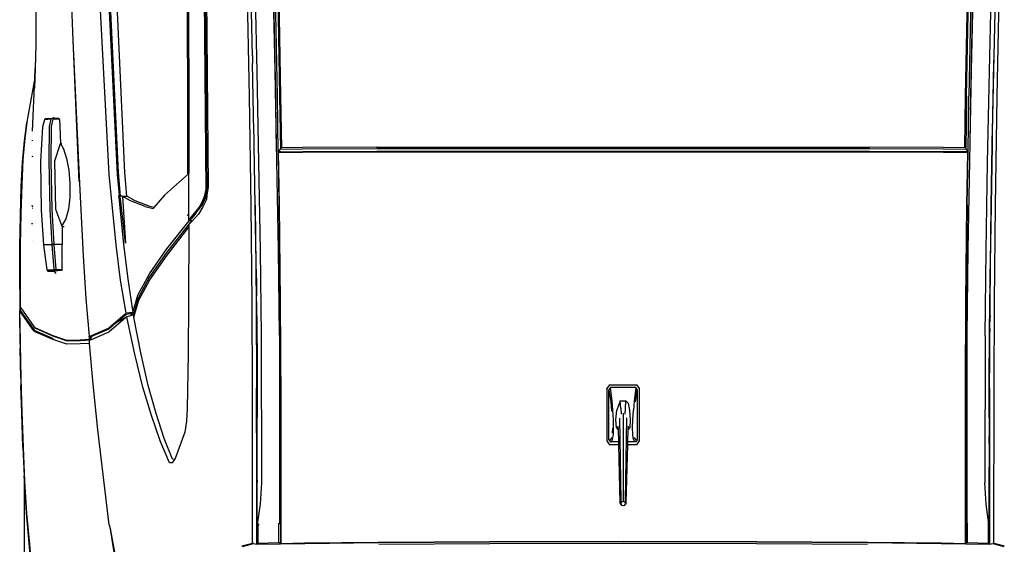
# Model space of a CAD drawing. Units: inches. Extents: x 22042254 to 25404563, y 17568978 to 17626777.
# Tile 26 of 45: x 22179810 to 22179874, y 17626227 to 17626261. Entities that reach past the tile are written whole.
import ezdxf

# ---------------------------------------------------------------- set-up
doc = ezdxf.new("R2010")
doc.units = ezdxf.units.IN
doc.header["$MEASUREMENT"] = 0
doc.layers.add('A-SITE-VEHI', color=8, linetype='Continuous', lineweight=18)
doc.layers.add('Edges', color=250, linetype='Continuous')

# ---------------------------------------------------------------- blocks, each defined once
blk = doc.blocks.new('Nissan Qashqai pl')
at = {"layer": 'Edges'}
for p, q in [((11.0581, 12.4738), (11.0614, 12.4872)), ((11.0582, 12.47), (11.0624, 12.4866)), ((10.3586, 12.4651), (10.2201, 12.4683)), ((10.2203, 12.4743), (10.3353, 12.4717)), ((10.2211, 12.4795), (10.3955, 12.4762)), ((10.3353, 12.4717), (10.4477, 12.4694)), ((10.3353, 12.4717), (10.346, 12.4714)), ((10.346, 12.4714), (10.4477, 12.4694)), ((10.3955, 12.4762), (10.5572, 12.4737)), ((10.4477, 12.4694), (10.4538, 12.4693)), ((10.4538, 12.4693), (10.4681, 12.469)), ((10.4676, 12.4691), (10.4538, 12.4693)), ((10.5566, 12.4677), (10.4676, 12.4691)), ((10.4676, 12.4691), (10.546, 12.4677)), ((10.4681, 12.469), (10.5866, 12.467)), ((10.546, 12.4677), (10.546, 12.4678)), ((10.546, 12.4677), (10.5576, 12.4675)), ((10.7, 12.4662), (10.5566, 12.4677)), ((10.5572, 12.4737), (10.7004, 12.4722)), ((10.5576, 12.4675), (10.6649, 12.4659)), ((10.5866, 12.467), (10.6649, 12.4659)), ((10.7004, 12.4722), (10.8279, 12.4715)), ((10.8279, 12.4715), (11.0544, 12.4714)), ((11.0544, 12.4714), (11.0575, 12.4714)), ((11.0575, 12.4714), (11.0581, 12.4738)), ((11.0575, 12.4714), (11.0582, 12.47)), ((11.0592, 12.4653), (11.0582, 12.47)), ((10.4931, 12.4624), (10.3586, 12.4651)), ((10.6237, 12.4603), (10.4931, 12.4624)), ((10.7502, 12.4586), (10.6237, 12.4603)), ((10.6649, 12.4659), (10.6786, 12.4658)), ((10.6649, 12.4659), (10.6772, 12.4657)), ((10.6786, 12.4657), (10.6772, 12.4657)), ((10.6786, 12.4658), (10.6786, 12.4662)), ((10.6786, 12.4657), (10.6786, 12.4658)), ((10.6786, 12.4658), (10.6801, 12.4657)), ((10.6786, 12.4657), (10.6801, 12.4657)), ((10.6801, 12.4662), (10.6801, 12.4657)), ((10.6801, 12.4657), (10.6801, 12.4657)), ((10.6801, 12.4657), (10.6811, 12.4657)), ((10.6801, 12.4657), (10.6811, 12.4657)), ((10.6811, 12.4662), (10.6811, 12.4657)), ((10.6811, 12.4657), (10.6811, 12.4657)), ((10.6811, 12.4657), (10.6966, 12.4654)), ((10.6811, 12.4657), (10.6991, 12.4655)), ((10.6811, 12.4657), (10.6991, 12.4655)), ((10.6966, 12.4654), (10.7144, 12.4653)), ((10.6991, 12.4655), (10.7144, 12.4653)), ((10.7201, 12.4661), (10.7, 12.4662)), ((10.7144, 12.4653), (10.7239, 12.4653)), ((10.7201, 12.4661), (10.7306, 12.4653)), ((10.7395, 12.4659), (10.7201, 12.4661)), ((10.7239, 12.4653), (10.7248, 12.4653)), ((10.7306, 12.4653), (10.7248, 12.4653)), ((10.7311, 12.4652), (10.7306, 12.4653)), ((10.7495, 12.4652), (10.7311, 12.4652)), ((10.7311, 12.4652), (10.7502, 12.4651)), ((10.7395, 12.4659), (10.7495, 12.4652)), ((10.7923, 12.4656), (10.7395, 12.4659)), ((10.8179, 12.4648), (10.7495, 12.4652)), ((10.7502, 12.4651), (10.7504, 12.4651)), ((10.7502, 12.4586), (10.968, 12.4585)), ((10.7504, 12.4651), (10.7808, 12.4649)), ((10.7808, 12.4649), (10.8179, 12.4648)), ((10.7923, 12.4652), (10.7923, 12.4656)), ((10.7933, 12.4656), (10.7923, 12.4656)), ((10.7933, 12.4652), (10.7933, 12.4656)), ((10.804, 12.4656), (10.7933, 12.4656)), ((10.804, 12.4653), (10.804, 12.4656)), ((10.8075, 12.4655), (10.804, 12.4656)), ((10.8075, 12.4655), (10.8075, 12.4653)), ((10.811, 12.4655), (10.8075, 12.4655)), ((10.811, 12.4655), (10.811, 12.4653)), ((10.8145, 12.4655), (10.811, 12.4655)), ((10.8145, 12.4653), (10.8145, 12.4655)), ((10.8279, 12.4654), (10.8145, 12.4655)), ((10.8277, 12.4647), (10.8179, 12.4648)), ((10.8711, 12.4646), (10.8277, 12.4647)), ((10.8279, 12.4654), (11.0592, 12.4653)), ((10.8711, 12.4646), (10.8824, 12.4646)), ((10.8824, 12.4646), (10.8825, 12.4646)), ((10.8825, 12.4646), (10.8884, 12.4646)), ((10.8884, 12.4646), (10.8923, 12.4646)), ((10.8923, 12.4646), (10.8996, 12.4646)), ((10.9097, 12.4646), (10.8996, 12.4646)), ((10.9097, 12.4646), (10.9399, 12.4646)), ((10.9399, 12.4646), (10.9491, 12.4645)), ((10.9491, 12.4645), (11.0301, 12.4645)), ((11, 12.4605), (10.968, 12.4585)), ((11.0301, 12.4645), (11, 12.4605)), ((11.0301, 12.4637), (11.0287, 12.4637)), ((11.03, 12.4635), (11.0301, 12.4637)), ((11.0301, 12.4642), (11.0301, 12.4645)), ((11.0574, 12.4637), (11.0301, 12.4637)), ((11.0568, 12.4323), (11.0574, 12.4637)), ((11.0574, 12.4637), (11.0592, 12.4653)), ((11.0585, 12.43), (11.0592, 12.4653)), ((10.2175, 12.4413), (10.3564, 12.4382)), ((10.2215, 12.4381), (10.3945, 12.4348)), ((10.2216, 12.4404), (10.3947, 12.4371)), ((10.3564, 12.4382), (10.4638, 12.436)), ((10.3947, 12.4314), (10.2218, 12.4347)), ((10.2218, 12.4327), (10.3947, 12.4294)), ((10.4773, 12.4335), (10.3945, 12.4348)), ((10.3947, 12.4371), (10.4638, 12.436)), ((10.3947, 12.4314), (10.4735, 12.4301)), ((10.3947, 12.4294), (10.4715, 12.4282)), ((10.4638, 12.436), (10.4914, 12.4355)), ((10.4715, 12.4282), (10.4711, 12.3973)), ((10.4731, 12.3973), (10.4735, 12.4301)), ((10.4735, 12.4301), (10.4773, 12.4335)), ((10.4773, 12.4296), (10.4769, 12.3968)), ((10.4773, 12.4335), (10.4773, 12.4296)), ((10.4785, 12.433), (10.4773, 12.4335)), ((10.5561, 12.4323), (10.4773, 12.4335)), ((10.4781, 12.3972), (10.4785, 12.433)), ((10.5563, 12.4318), (10.4785, 12.433)), ((10.4914, 12.4355), (10.6223, 12.4333)), ((10.5561, 12.4323), (10.6996, 12.4308)), ((10.6999, 12.4304), (10.5563, 12.4318)), ((10.6223, 12.4333), (10.7493, 12.4316)), ((10.6996, 12.4308), (10.7722, 12.4304)), ((10.827, 12.4297), (10.6999, 12.4304)), ((10.7493, 12.4316), (11.0294, 12.4315)), ((10.7722, 12.4304), (10.7722, 12.4302)), ((10.7722, 12.4304), (10.7889, 12.4303)), ((10.7889, 12.4302), (10.7889, 12.4303)), ((10.7889, 12.4303), (10.7923, 12.4303)), ((10.7923, 12.4302), (10.7923, 12.4303)), ((10.7923, 12.4303), (10.7933, 12.4303)), ((10.7933, 12.4302), (10.7933, 12.4303)), ((10.7933, 12.4303), (10.8267, 12.4301)), ((10.8267, 12.4301), (11.0585, 12.43)), ((10.9133, 12.4296), (10.827, 12.4297)), ((10.9133, 12.4296), (10.9133, 12.4298)), ((10.9137, 12.4296), (10.9133, 12.4296)), ((10.9137, 12.4296), (10.9138, 12.4298)), ((10.9715, 12.4296), (10.9137, 12.4296)), ((10.9715, 12.4299), (10.9715, 12.4296)), ((11.0579, 12.4296), (10.9715, 12.4296)), ((11.0281, 12.4323), (11.0568, 12.4323)), ((11.0294, 12.4315), (11.0294, 12.4316)), ((11.0295, 12.4341), (11.0295, 12.4343)), ((11.0568, 12.4323), (11.0585, 12.43)), ((11.0572, 12.3942), (11.0579, 12.4296)), ((11.0579, 12.3938), (11.0585, 12.43)), ((11.0579, 12.4296), (11.0585, 12.43)), ((10.4711, 12.3973), (10.4706, 12.2875)), ((10.4726, 12.2875), (10.4731, 12.3973)), ((10.4764, 12.2872), (10.4769, 12.3968)), ((10.4776, 12.2874), (10.4781, 12.3972)), ((11.056, 12.2851), (11.0572, 12.3942)), ((11.0566, 12.2849), (11.0579, 12.3938)), ((10.4706, 11.5566), (10.4706, 12.2875)), ((10.4726, 11.5567), (10.4726, 12.2875)), ((10.4764, 11.5569), (10.4764, 12.2872)), ((10.4776, 11.5567), (10.4776, 12.2874)), ((11.0551, 12.1203), (11.056, 12.2851)), ((11.0557, 12.1202), (11.0566, 12.2849)), ((11.0595, 12.2842), (11.0586, 12.1198)), ((11.0547, 11.9221), (11.0551, 12.1203)), ((11.0554, 11.9221), (11.0557, 12.1202)), ((11.0586, 12.1198), (11.0583, 11.9221)), ((10.8228, 11.9421), (10.8224, 11.9421)), ((10.8228, 11.9421), (10.8283, 11.9461)), ((10.8228, 11.9021), (10.8228, 11.9421)), ((10.827, 11.9408), (10.8301, 11.9431)), ((10.8279, 11.9461), (10.8283, 11.9461)), ((10.8283, 11.9461), (10.906, 11.9461)), ((10.8483, 11.9406), (10.8301, 11.9431)), ((10.8301, 11.9431), (10.9043, 11.9431)), ((10.905, 11.9414), (10.9035, 11.9403)), ((10.9043, 11.9431), (10.9074, 11.9408)), ((10.9043, 11.9431), (10.905, 11.9414)), ((10.906, 11.9461), (10.9116, 11.9421)), ((10.9116, 11.9421), (10.9116, 11.929)), ((10.827, 11.9408), (10.827, 11.9033)), ((10.827, 11.9408), (10.8467, 11.9386)), ((10.8467, 11.9386), (10.8603, 11.9373)), ((10.8467, 11.9263), (10.8501, 11.9295)), ((10.8501, 11.9295), (10.8603, 11.9316)), ((10.8746, 11.9363), (10.8603, 11.9373)), ((10.8603, 11.9316), (10.8746, 11.9327)), ((10.9946, 11.9254), (10.872, 11.9276)), ((10.8861, 11.9361), (10.8746, 11.9363)), ((10.8746, 11.9327), (10.8861, 11.9319)), ((10.889, 11.9296), (10.884, 11.9298)), ((10.8959, 11.9365), (10.8861, 11.9361)), ((10.8861, 11.9319), (10.889, 11.9296)), ((10.9074, 11.9291), (10.889, 11.9296)), ((10.9021, 11.9372), (10.8959, 11.9365)), ((10.9035, 11.9403), (10.9008, 11.9391)), ((10.9057, 11.9384), (10.9021, 11.9372)), ((10.9074, 11.9393), (10.9057, 11.9384)), ((10.9074, 11.9408), (10.9074, 11.9393)), ((10.9074, 11.9393), (10.9074, 11.9291)), ((10.9116, 11.929), (10.9074, 11.9291)), ((10.9973, 11.9268), (10.9116, 11.929)), ((10.9973, 11.9268), (11.0001, 11.9254)), ((10.999, 11.9258), (10.9973, 11.9268)), ((10.8467, 11.9178), (10.8467, 11.9263)), ((10.8579, 11.9255), (10.8467, 11.9263)), ((10.8579, 11.9187), (10.8467, 11.9178)), ((10.8467, 11.9178), (10.8603, 11.9126)), ((10.8662, 11.925), (10.8579, 11.9255)), ((10.8579, 11.9187), (10.8662, 11.9191)), ((10.8746, 11.9115), (10.8603, 11.9126)), ((10.8647, 11.9221), (10.996, 11.9221)), ((10.8723, 11.9165), (10.9946, 11.9187)), ((10.8861, 11.9122), (10.8746, 11.9115)), ((10.884, 11.9144), (10.889, 11.9145)), ((10.889, 11.9145), (10.8861, 11.9122)), ((10.889, 11.9145), (10.9074, 11.915)), ((10.9074, 11.915), (10.9116, 11.9151)), ((10.9074, 11.915), (10.9074, 11.9049)), ((10.9116, 11.9151), (10.9973, 11.9173)), ((10.9116, 11.9151), (10.9116, 11.9021)), ((10.9969, 11.9247), (10.9946, 11.9254)), ((10.9946, 11.9187), (10.9969, 11.9195)), ((10.9969, 11.9247), (10.996, 11.9221)), ((10.996, 11.9221), (10.9969, 11.9195)), ((10.999, 11.9258), (10.9969, 11.9247)), ((10.9969, 11.9195), (10.999, 11.9184)), ((11.0001, 11.9187), (10.9973, 11.9173)), ((10.9973, 11.9173), (10.999, 11.9184)), ((11.0012, 11.9247), (10.999, 11.9258)), ((10.999, 11.9184), (10.9996, 11.9187)), ((10.9996, 11.9187), (11.0012, 11.9195)), ((11.0001, 11.9187), (10.9996, 11.9187)), ((11.0012, 11.9247), (11.0001, 11.9254)), ((11.0012, 11.9195), (11.0001, 11.9187)), ((11.002, 11.9221), (11.0012, 11.9247)), ((11.0012, 11.9195), (11.002, 11.9221)), ((11.0551, 11.7239), (11.0547, 11.9221)), ((11.0557, 11.724), (11.0554, 11.9221)), ((11.0583, 11.9221), (11.0586, 11.7244)), ((10.8224, 11.9021), (10.8228, 11.9021)), ((10.8228, 11.9021), (10.8283, 11.8981)), ((10.8467, 11.9056), (10.827, 11.9033)), ((10.827, 11.9033), (10.8301, 11.9011)), ((10.8283, 11.8981), (10.8279, 11.8981)), ((10.8283, 11.8981), (10.906, 11.8981)), ((10.8301, 11.9011), (10.8483, 11.9036)), ((10.9043, 11.9011), (10.8301, 11.9011)), ((10.8603, 11.9068), (10.8467, 11.9056)), ((10.8483, 11.9036), (10.8619, 11.905)), ((10.8746, 11.9078), (10.8603, 11.9068)), ((10.8861, 11.908), (10.8746, 11.9078)), ((10.8959, 11.9077), (10.8861, 11.908)), ((10.8871, 11.9063), (10.8944, 11.906)), ((10.9021, 11.9069), (10.8959, 11.9077)), ((10.9008, 11.905), (10.9035, 11.9039)), ((10.9057, 11.9058), (10.9021, 11.9069)), ((10.9035, 11.9039), (10.905, 11.9028)), ((10.9043, 11.9011), (10.9074, 11.9033)), ((10.905, 11.9028), (10.9043, 11.9011)), ((10.9074, 11.9049), (10.9057, 11.9058)), ((10.906, 11.8981), (10.9116, 11.9021)), ((10.9074, 11.9033), (10.9074, 11.9049)), ((10.9074, 11.9033), (10.9074, 11.9048)), ((11.056, 11.559), (11.0551, 11.7239)), ((11.0566, 11.5593), (11.0557, 11.724)), ((11.0586, 11.7244), (11.0595, 11.5599)), ((10.4706, 11.5566), (10.4711, 11.4469)), ((10.4731, 11.4469), (10.4726, 11.5567)), ((10.4769, 11.4474), (10.4764, 11.5569)), ((10.4781, 11.4469), (10.4776, 11.5567)), ((11.0572, 11.4499), (11.056, 11.559)), ((11.0579, 11.4504), (11.0566, 11.5593)), ((10.4711, 11.4469), (10.4715, 11.416)), ((10.4735, 11.414), (10.4731, 11.4469)), ((10.4773, 11.4146), (10.4769, 11.4474)), ((10.4785, 11.4111), (10.4781, 11.4469)), ((11.0579, 11.4146), (11.0572, 11.4499)), ((11.0585, 11.4142), (11.0579, 11.4504)), ((10.4715, 11.416), (10.3947, 11.4148)), ((10.3564, 11.406), (10.2175, 11.4028)), ((10.3945, 11.4094), (10.2215, 11.406)), ((10.3947, 11.4071), (10.2216, 11.4037)), ((10.3947, 11.4148), (10.2218, 11.4114)), ((10.2218, 11.4094), (10.3947, 11.4128)), ((10.4416, 11.4077), (10.3564, 11.406)), ((10.4773, 11.4107), (10.3945, 11.4094)), ((10.3947, 11.4128), (10.4735, 11.414)), ((10.4416, 11.4078), (10.3947, 11.4071)), ((10.4519, 11.4079), (10.4416, 11.4077)), ((10.4519, 11.4079), (10.4416, 11.4078)), ((10.4416, 11.4077), (10.4416, 11.4078)), ((10.4524, 11.408), (10.4519, 11.4079)), ((10.4519, 11.4079), (10.4519, 11.4079)), ((10.4524, 11.4079), (10.4519, 11.4079)), ((10.4524, 11.4079), (10.4524, 11.408)), ((10.4533, 11.408), (10.4524, 11.408)), ((10.4533, 11.4079), (10.4524, 11.4079)), ((10.4638, 11.4081), (10.4533, 11.4079)), ((10.4638, 11.4081), (10.4533, 11.408)), ((10.4533, 11.4079), (10.4533, 11.408)), ((10.4914, 11.4087), (10.4638, 11.4081)), ((10.4773, 11.4107), (10.4735, 11.414)), ((10.4773, 11.4146), (10.4773, 11.4107)), ((10.4773, 11.4107), (10.5561, 11.4119)), ((10.4773, 11.4107), (10.4785, 11.4111)), ((10.5563, 11.4123), (10.4785, 11.4111)), ((10.6223, 11.4109), (10.4914, 11.4087)), ((10.6996, 11.4134), (10.5561, 11.4119)), ((10.5563, 11.4123), (10.6999, 11.4138)), ((10.7493, 11.4125), (10.6223, 11.4109)), ((10.7722, 11.4138), (10.6996, 11.4134)), ((10.6999, 11.4138), (10.7722, 11.4142)), ((10.7493, 11.4125), (11.0294, 11.4126)), ((10.7722, 11.4142), (10.7889, 11.4143)), ((10.7722, 11.4142), (10.7722, 11.4138)), ((10.7889, 11.4139), (10.7722, 11.4138)), ((10.7889, 11.4139), (10.7889, 11.4143)), ((10.7889, 11.4143), (10.7923, 11.4143)), ((10.7923, 11.4139), (10.7889, 11.4139)), ((10.7923, 11.4139), (10.7923, 11.4143)), ((10.7923, 11.4143), (10.7933, 11.4143)), ((10.7933, 11.4139), (10.7923, 11.4139)), ((10.7933, 11.4143), (10.827, 11.4145)), ((10.7933, 11.4139), (10.7933, 11.4143)), ((10.8267, 11.4141), (10.7933, 11.4139)), ((10.8267, 11.4141), (11.0585, 11.4142)), ((10.827, 11.4145), (11.0579, 11.4146)), ((11.0294, 11.4118), (11.0281, 11.4118)), ((11.0294, 11.4125), (11.0294, 11.4126)), ((11.0295, 11.4116), (11.0294, 11.4118)), ((11.0568, 11.4118), (11.0294, 11.4118)), ((11.0585, 11.4142), (11.0568, 11.4118)), ((11.0574, 11.3804), (11.0568, 11.4118)), ((11.0585, 11.4142), (11.0579, 11.4146)), ((11.0592, 11.3789), (11.0585, 11.4142)), ((10.2201, 11.3759), (10.3586, 11.3791)), ((10.3353, 11.3725), (10.2203, 11.3699)), ((10.3353, 11.3725), (10.346, 11.3727)), ((10.4477, 11.3747), (10.346, 11.3727)), ((10.3586, 11.3791), (10.4931, 11.3817)), ((10.4537, 11.3749), (10.4477, 11.3747)), ((10.4537, 11.3749), (10.4538, 11.3749)), ((10.4681, 11.3752), (10.4538, 11.3749)), ((10.4676, 11.3751), (10.4538, 11.3749)), ((10.5576, 11.3766), (10.4676, 11.3751)), ((10.5566, 11.3765), (10.4676, 11.3751)), ((10.4676, 11.3751), (10.4676, 11.3751)), ((10.5866, 11.3772), (10.4681, 11.3752)), ((10.4931, 11.3817), (10.6237, 11.3839)), ((10.5566, 11.3765), (10.7, 11.378)), ((10.6649, 11.3783), (10.5576, 11.3766)), ((10.6649, 11.3783), (10.5866, 11.3772)), ((10.6237, 11.3839), (10.7502, 11.3855)), ((10.6908, 11.3785), (10.6649, 11.3783)), ((10.6649, 11.3783), (10.6772, 11.3784)), ((10.6966, 11.3787), (10.6772, 11.3784)), ((10.6772, 11.3784), (10.6908, 11.3785)), ((10.6991, 11.3786), (10.6908, 11.3785)), ((10.7144, 11.3788), (10.6966, 11.3787)), ((10.6999, 11.3786), (10.6991, 11.3786)), ((10.6999, 11.3786), (10.7808, 11.3793)), ((10.7144, 11.3788), (10.6999, 11.3786)), ((10.7, 11.378), (10.8279, 11.3787)), ((10.8279, 11.3727), (10.7004, 11.372)), ((10.7239, 11.3789), (10.7144, 11.3788)), ((10.7248, 11.3789), (10.7239, 11.3789)), ((10.7808, 11.3793), (10.7248, 11.3789)), ((10.7502, 11.3855), (10.968, 11.3857)), ((10.7808, 11.3793), (10.8711, 11.3796)), ((10.9431, 11.3796), (10.8279, 11.3787)), ((10.8279, 11.3787), (11.0552, 11.3789)), ((10.9614, 11.3788), (10.8279, 11.3787)), ((11.0544, 11.3728), (10.8279, 11.3727)), ((10.896, 11.3796), (10.8711, 11.3796)), ((10.9097, 11.3796), (10.896, 11.3796)), ((10.9431, 11.3796), (10.9097, 11.3796)), ((10.9478, 11.3796), (10.9431, 11.3796)), ((10.9491, 11.3796), (10.9478, 11.3796)), ((10.9668, 11.3796), (10.9491, 11.3796)), ((10.9614, 11.3788), (10.9668, 11.3796)), ((10.9711, 11.3788), (10.9614, 11.3788)), ((10.9668, 11.3796), (10.967, 11.3796)), ((10.9765, 11.3796), (10.967, 11.3796)), ((10.968, 11.3857), (11, 11.3837)), ((10.9765, 11.3796), (10.9711, 11.3788)), ((10.9766, 11.3788), (10.9711, 11.3788)), ((10.9765, 11.3796), (10.9766, 11.3788)), ((10.9825, 11.3796), (10.9765, 11.3796)), ((11.0592, 11.3789), (10.9766, 11.3788)), ((11.0301, 11.3796), (10.9825, 11.3796)), ((11, 11.3837), (11.0301, 11.3796)), ((11.0287, 11.3804), (11.0301, 11.3804)), ((11.0301, 11.3803), (11.0292, 11.3802)), ((11.03, 11.3822), (11.03, 11.3824)), ((11.0301, 11.3803), (11.0301, 11.3804)), ((11.0301, 11.3804), (11.0554, 11.3804)), ((11.0554, 11.3804), (11.0301, 11.3803)), ((11.0301, 11.3796), (11.0301, 11.3803)), ((11.0575, 11.3728), (11.0544, 11.3728)), ((11.0554, 11.3804), (11.0574, 11.3804)), ((11.0592, 11.3789), (11.0574, 11.3804)), ((11.0582, 11.3742), (11.0575, 11.3728)), ((11.0581, 11.3704), (11.0575, 11.3728)), ((11.0582, 11.3742), (11.0592, 11.3789)), ((11.0624, 11.3576), (11.0582, 11.3742)), ((10.3955, 11.368), (10.2211, 11.3646)), ((10.5572, 11.3704), (10.3955, 11.368)), ((10.7004, 11.372), (10.5572, 11.3704)), ((11.0614, 11.3569), (11.0581, 11.3704)), ((10.2357, 11.3043), (10.53, 11.3068)), ((10.2367, 11.3022), (10.5351, 11.305)), ((10.2369, 11.3008), (10.5348, 11.3036)), ((10.4153, 11.3058), (10.2954, 11.3046)), ((10.4153, 11.3058), (10.4174, 11.3058)), ((10.4174, 11.3058), (10.4181, 11.3058)), ((10.4181, 11.3058), (10.4182, 11.3058)), ((10.4182, 11.3058), (10.53, 11.3068)), ((10.53, 11.3068), (10.5301, 11.3068)), ((10.5301, 11.3068), (10.5323, 11.3065)), ((10.5323, 11.3065), (10.5419, 11.3051)), ((10.5422, 11.3021), (10.5348, 11.3036)), ((10.5424, 11.3035), (10.5351, 11.305)), ((10.5366, 11.3048), (10.536, 11.305)), ((10.5379, 11.3052), (10.5381, 11.305)), ((10.5419, 11.3051), (10.5463, 11.3031)), ((10.5419, 11.3051), (10.5479, 11.3042)), ((10.5522, 11.2977), (10.5422, 11.3021)), ((10.5472, 11.3014), (10.5424, 11.3035)), ((10.5463, 11.3031), (10.5551, 11.2984)), ((10.5546, 11.2982), (10.5472, 11.3014)), ((10.5479, 11.3042), (10.5589, 11.2991)), ((10.5589, 11.2991), (10.57, 11.2925)), ((10.5598, 11.2935), (10.5522, 11.2977)), ((10.5583, 11.296), (10.5546, 11.2982)), ((10.5551, 11.2984), (10.5583, 11.296)), ((10.5612, 11.2944), (10.5583, 11.296)), ((10.5764, 11.28), (10.5598, 11.2935)), ((10.5683, 11.2885), (10.5612, 11.2944)), ((10.5683, 11.2885), (10.573, 11.285)), ((10.575, 11.2829), (10.5683, 11.2885)), ((10.57, 11.2925), (10.5811, 11.2822)), ((10.573, 11.285), (10.5769, 11.2818)), ((10.2453, 11.2777), (10.4289, 11.2783)), ((10.4292, 11.2767), (10.2453, 11.2762)), ((10.4289, 11.2783), (10.5092, 11.2783)), ((10.5099, 11.2768), (10.4292, 11.2767)), ((10.5099, 11.2768), (10.5092, 11.2783)), ((10.5092, 11.2783), (10.5094, 11.2783)), ((10.5094, 11.2783), (10.51, 11.2776)), ((10.5783, 11.2783), (10.5094, 11.2783)), ((10.51, 11.2776), (10.5099, 11.2768)), ((10.51, 11.2776), (10.5419, 11.2423)), ((10.5705, 11.2771), (10.5709, 11.2767)), ((10.5709, 11.2767), (10.5719, 11.2759)), ((10.5776, 11.2808), (10.575, 11.2829)), ((10.5783, 11.2783), (10.5764, 11.28)), ((10.5796, 11.2787), (10.5776, 11.2808)), ((10.5776, 11.2808), (10.5783, 11.2783)), ((10.5796, 11.2787), (10.5783, 11.2783)), ((10.5796, 11.2824), (10.5796, 11.2787)), ((10.6215, 11.2456), (10.5796, 11.2787)), ((10.5811, 11.2822), (10.5821, 11.2808)), ((10.5811, 11.2822), (10.5834, 11.28)), ((10.5821, 11.2808), (10.5834, 11.2793)), ((10.5825, 11.2806), (10.5834, 11.2793)), ((10.5834, 11.28), (10.5851, 11.2783)), ((10.5834, 11.2793), (10.5835, 11.2793)), ((10.5835, 11.2793), (10.584, 11.2787)), ((10.584, 11.2789), (10.584, 11.2793)), ((10.584, 11.2787), (10.584, 11.2789)), ((10.584, 11.2787), (10.6261, 11.2458)), ((10.584, 11.2787), (10.5851, 11.2783)), ((10.5843, 11.2787), (10.584, 11.2787)), ((10.5847, 11.2787), (10.5843, 11.2787)), ((10.5851, 11.2783), (10.5892, 11.2783)), ((10.6306, 11.2459), (10.5892, 11.2783)), ((10.5892, 11.2783), (10.6988, 11.2779)), ((10.6988, 11.2779), (10.7769, 11.2774)), ((10.7769, 11.2774), (10.858, 11.2759)), ((10.858, 11.2759), (10.8766, 11.2745)), ((10.8766, 11.2745), (10.8932, 11.2722)), ((10.8932, 11.2722), (10.932, 11.258)), ((10.932, 11.258), (10.9335, 11.257)), ((10.9335, 11.257), (10.933, 11.2541)), ((10.9335, 11.257), (10.9386, 11.2537)), ((10.5419, 11.2423), (10.56, 11.2265)), ((10.6583, 11.2197), (10.6215, 11.2456)), ((10.6261, 11.2458), (10.6627, 11.22)), ((10.6671, 11.2203), (10.6306, 11.2459)), ((10.9026, 11.2417), (10.8653, 11.2297)), ((10.933, 11.2541), (10.9026, 11.2417)), ((10.9384, 11.2497), (10.9059, 11.2355)), ((10.9386, 11.2537), (10.9384, 11.2497)), ((10.56, 11.2265), (10.5584, 11.2206)), ((10.56, 11.2265), (10.5617, 11.2251)), ((10.8653, 11.2297), (10.8239, 11.2181)), ((10.9059, 11.2355), (10.8682, 11.2226)), ((10.5584, 11.2206), (10.5502, 11.1986)), ((10.5584, 11.2136), (10.5502, 11.1916)), ((10.5584, 11.2136), (10.5617, 11.2251)), ((10.69, 11.2028), (10.6583, 11.2197)), ((10.6627, 11.22), (10.6943, 11.2032)), ((10.6976, 11.2041), (10.6671, 11.2203)), ((10.8239, 11.2181), (10.7754, 11.2071)), ((10.8682, 11.2226), (10.8264, 11.21)), ((10.5502, 11.1986), (10.543, 11.1865)), ((10.7155, 11.1952), (10.69, 11.2028)), ((10.6943, 11.2032), (10.7155, 11.1969)), ((10.7228, 11.1965), (10.6976, 11.2041)), ((10.7155, 11.1957), (10.7155, 11.1969)), ((10.7155, 11.1969), (10.7192, 11.1957)), ((10.7754, 11.2071), (10.7228, 11.1965)), ((10.7776, 11.1982), (10.7247, 11.1867)), ((10.8264, 11.21), (10.7776, 11.1982)), ((10.5079, 11.1835), (10.1849, 11.1687)), ((10.543, 11.1865), (10.5079, 11.1835)), ((10.5502, 11.1916), (10.543, 11.1795)), ((10.543, 11.1795), (10.543, 11.1865)), ((10.5439, 11.1796), (10.613, 11.1841)), ((10.613, 11.1841), (10.547, 11.1767)), ((10.6144, 11.1813), (10.6664, 11.1875)), ((10.6664, 11.1875), (10.7155, 11.1952)), ((10.7137, 11.1846), (10.6678, 11.177)), ((10.7165, 11.1851), (10.7137, 11.1846)), ((10.7209, 11.1902), (10.7155, 11.1957)), ((10.7155, 11.1952), (10.7155, 11.1957)), ((10.7186, 11.1848), (10.7155, 11.1952)), ((10.7155, 11.1952), (10.7165, 11.1851)), ((10.7177, 11.1838), (10.7165, 11.1851)), ((10.7387, 11.1593), (10.7177, 11.1838)), ((10.7312, 11.1701), (10.7186, 11.1848)), ((10.7192, 11.1957), (10.7228, 11.1965)), ((10.7192, 11.1957), (10.7209, 11.1902)), ((10.7209, 11.1902), (10.7221, 11.1861)), ((10.7221, 11.1861), (10.7222, 11.1859)), ((10.7222, 11.186), (10.7221, 11.1861)), ((10.7247, 11.1867), (10.7222, 11.186)), ((10.7222, 11.186), (10.7222, 11.1859)), ((10.7222, 11.1859), (10.7232, 11.1848)), ((10.7222, 11.1859), (10.7224, 11.1855)), ((10.7224, 11.1855), (10.7312, 11.1701)), ((10.7232, 11.1848), (10.7228, 11.1859)), ((10.7232, 11.1848), (10.7449, 11.1598)), ((10.7257, 11.1853), (10.7256, 11.1854)), ((11.0357, 11.1613), (11.1598, 11.1847)), ((10.5079, 11.1739), (10.1849, 11.1585)), ((10.1894, 11.1563), (10.5109, 11.1721)), ((10.543, 11.1771), (10.5079, 11.1739)), ((10.5109, 11.1721), (10.5417, 11.1748)), ((10.6152, 11.1702), (10.5113, 11.1603)), ((10.543, 11.1771), (10.5417, 11.1748)), ((10.5417, 11.1748), (10.5427, 11.1739)), ((10.5436, 11.1754), (10.5427, 11.1739)), ((10.5427, 11.1739), (10.5458, 11.1742)), ((10.5439, 11.1796), (10.543, 11.1795)), ((10.543, 11.1795), (10.543, 11.1771)), ((10.544, 11.1763), (10.543, 11.1771)), ((10.544, 11.1763), (10.5436, 11.1754)), ((10.547, 11.1767), (10.544, 11.1763)), ((10.5458, 11.1742), (10.6144, 11.1813)), ((10.6678, 11.177), (10.6152, 11.1702)), ((10.7397, 11.1602), (10.7312, 11.1701)), ((11.0492, 11.1635), (11.1336, 11.1772)), ((10.5113, 11.1603), (10.19, 11.1433)), ((10.7501, 11.1327), (10.7387, 11.1593)), ((10.7507, 11.1344), (10.7397, 11.1602)), ((10.7449, 11.1598), (10.7563, 11.1333)), ((11.0304, 11.1603), (10.8896, 11.1434)), ((11.0304, 11.1603), (11.0357, 11.1613)), ((11.0357, 11.1613), (11.0491, 11.1635)), ((11.0492, 11.1635), (11.0491, 11.1635)), ((10.8896, 11.1434), (10.8218, 11.1365)), ((10.6318, 11.1213), (10.6955, 11.1257)), ((10.6955, 11.1257), (10.7509, 11.1302)), ((10.7507, 11.1309), (10.7501, 11.1327)), ((10.7511, 11.1335), (10.7507, 11.1344)), ((10.7507, 11.1344), (10.7524, 11.1335)), ((10.751, 11.131), (10.7507, 11.1309)), ((10.7509, 11.1302), (10.7507, 11.1309)), ((10.7522, 11.1311), (10.7509, 11.1302)), ((10.7516, 11.131), (10.7509, 11.1302)), ((10.7519, 11.1314), (10.7511, 11.1335)), ((10.7519, 11.1314), (10.7516, 11.131)), ((10.7522, 11.1311), (10.7516, 11.131)), ((10.7526, 11.1318), (10.7519, 11.1314)), ((10.7553, 11.1307), (10.7522, 11.1311)), ((10.7524, 11.1335), (10.7526, 11.1318)), ((10.7524, 11.1335), (10.7556, 11.1319)), ((10.7532, 11.1321), (10.7526, 11.1318)), ((10.7526, 11.1318), (10.7526, 11.1314)), ((10.7556, 11.1319), (10.7532, 11.1321)), ((10.7563, 11.1169), (10.7553, 11.1307)), ((10.7556, 11.1319), (10.7561, 11.1317)), ((10.7563, 11.1319), (10.7561, 11.1319)), ((10.7563, 11.1315), (10.7561, 11.1317)), ((10.7561, 11.1317), (10.7563, 11.1317)), ((10.7563, 11.1333), (10.7569, 11.1317)), ((10.7563, 11.1317), (10.7563, 11.1319)), ((10.7563, 11.1317), (10.7569, 11.1317)), ((10.7569, 11.1316), (10.7563, 11.1317)), ((10.7563, 11.1315), (10.7563, 11.1317)), ((10.7572, 11.1178), (10.7563, 11.1315)), ((10.7573, 11.1307), (10.7563, 11.1315)), ((10.7569, 11.1317), (10.7569, 11.1316)), ((10.7569, 11.1316), (10.7573, 11.1307)), ((10.7604, 11.131), (10.7573, 11.1307)), ((10.7615, 11.1311), (10.7604, 11.131)), ((10.8218, 11.1365), (10.7615, 11.1311)), ((10.7615, 11.1311), (10.7623, 11.1173)), ((10.312, 11.1064), (10.5147, 11.1156)), ((10.312, 11.1064), (10.5214, 11.1149)), ((10.5147, 11.1156), (10.6318, 11.1213)), ((10.7565, 11.0969), (10.7563, 11.1169)), ((10.7575, 11.0979), (10.7572, 11.1178)), ((10.7623, 11.1173), (10.7626, 11.0974)), ((10.2081, 11.1017), (10.312, 11.1064)), ((10.4732, 11.0925), (10.4871, 11.0967)), ((10.4871, 11.0967), (10.5048, 11.1002)), ((10.5048, 11.1002), (10.5246, 11.1019)), ((10.5246, 11.1019), (10.5445, 11.1017)), ((10.5445, 11.1017), (10.5625, 11.0996)), ((10.5625, 11.0996), (10.5769, 11.0957)), ((10.5769, 11.0957), (10.5863, 11.0904)), ((10.7497, 11.0763), (10.7565, 11.0969)), ((10.7507, 11.0773), (10.7575, 11.0979)), ((10.7626, 11.0974), (10.7559, 11.0767)), ((10.4274, 11.0767), (10.4275, 11.0856)), ((10.4275, 11.0856), (10.4293, 11.0863)), ((10.4293, 11.0863), (10.4291, 11.0765)), ((10.4293, 11.0863), (10.4398, 11.0868)), ((10.4398, 11.0868), (10.4653, 11.0878)), ((10.4653, 11.0881), (10.4652, 11.0897)), ((10.4653, 11.0881), (10.4732, 11.0925)), ((10.4653, 11.0877), (10.4653, 11.0881)), ((10.4653, 11.0878), (10.4653, 11.0881)), ((10.4653, 11.0881), (10.4653, 11.0881)), ((10.4653, 11.0877), (10.4653, 11.0878)), ((10.4908, 11.0793), (10.4653, 11.0877)), ((10.563, 11.0809), (10.4908, 11.0793)), ((10.5867, 11.0897), (10.563, 11.0809)), ((10.5863, 11.0904), (10.5867, 11.0897)), ((10.5885, 11.0904), (10.5867, 11.0897)), ((10.5885, 11.0931), (10.5885, 11.0904)), ((10.5885, 11.0904), (10.6141, 11.0905)), ((10.6141, 11.0905), (10.615, 11.0905)), ((10.6142, 11.0782), (10.6141, 11.0905)), ((10.6517, 11.0902), (10.615, 11.0905)), ((10.615, 11.0905), (10.6151, 11.0782)), ((10.6151, 11.078), (10.6518, 11.0808)), ((10.6518, 11.0808), (10.6517, 11.0902)), ((10.6517, 11.0902), (10.6535, 11.0895)), ((10.6518, 11.0784), (10.6518, 11.0808)), ((10.6518, 11.0808), (10.6536, 11.0803)), ((10.6536, 11.0803), (10.6518, 11.0784)), ((10.6535, 11.0895), (10.6543, 11.0786)), ((10.6535, 11.0895), (10.6536, 11.0803)), ((10.6536, 11.0803), (10.6537, 11.0783)), ((10.6578, 11.0814), (10.6543, 11.0786)), ((10.4263, 11.0777), (10.4274, 11.0767)), ((10.4274, 11.0762), (10.4274, 11.0767)), ((10.4282, 11.0666), (10.4274, 11.0762)), ((10.4282, 11.0666), (10.4299, 11.0644)), ((10.4291, 11.0765), (10.4398, 11.0741)), ((10.4398, 11.0718), (10.4291, 11.0741)), ((10.4291, 11.0741), (10.4299, 11.0644)), ((10.4398, 11.0741), (10.4909, 11.0734)), ((10.4909, 11.0711), (10.4398, 11.0718)), ((10.4909, 11.0734), (10.563, 11.075)), ((10.5631, 11.0727), (10.4909, 11.0711)), ((10.563, 11.075), (10.6142, 11.0779)), ((10.6142, 11.0756), (10.5631, 11.0727)), ((10.6142, 11.0779), (10.6142, 11.0782)), ((10.6142, 11.0765), (10.6142, 11.0779)), ((10.615, 11.0765), (10.6142, 11.0765)), ((10.6142, 11.0756), (10.6142, 11.0765)), ((10.615, 11.0639), (10.6142, 11.0756)), ((10.6151, 11.0765), (10.615, 11.0765)), ((10.615, 11.0765), (10.6151, 11.0639)), ((10.6518, 11.0784), (10.6151, 11.0756)), ((10.6151, 11.0782), (10.6151, 11.078)), ((10.6151, 11.078), (10.6151, 11.0765)), ((10.6151, 11.0765), (10.6151, 11.0756)), ((10.6151, 11.0756), (10.616, 11.0629)), ((10.616, 11.0629), (10.6526, 11.0674)), ((10.6526, 11.0674), (10.6518, 11.0784)), ((10.6526, 11.0674), (10.6543, 11.0693)), ((10.6543, 11.0786), (10.6537, 11.0783)), ((10.6537, 11.0783), (10.6543, 11.0693)), ((10.6543, 11.0693), (10.6543, 11.0786)), ((10.7385, 11.051), (10.7497, 11.0763)), ((10.7396, 11.0519), (10.7507, 11.0773)), ((10.7549, 11.0776), (10.743, 11.0503)), ((10.7559, 11.0767), (10.7448, 11.0511)), ((10.2677, 11.0512), (10.3189, 11.0511)), ((10.3189, 11.0511), (10.3537, 11.0503)), ((10.4299, 11.0644), (10.4406, 11.0612)), ((10.4406, 11.0612), (10.4919, 11.0584)), ((10.4919, 11.0584), (10.564, 11.0591)), ((10.564, 11.0591), (10.6151, 11.0628)), ((10.6151, 11.0639), (10.615, 11.0639)), ((10.6151, 11.0628), (10.615, 11.0639)), ((10.6151, 11.0639), (10.6151, 11.0628)), ((10.7378, 11.0495), (10.7385, 11.051)), ((10.7387, 11.0502), (10.7396, 11.0519)), ((10.7448, 11.0511), (10.744, 11.0494)), ((10.3537, 11.0503), (10.3832, 11.0496)), ((10.3679, 11.0497), (10.3537, 11.0503)), ((10.3679, 11.0497), (10.4275, 11.0391)), ((10.4468, 11.0466), (10.3679, 11.0497)), ((10.4275, 11.0391), (10.4304, 11.0385)), ((10.4304, 11.0385), (10.4339, 11.0381)), ((10.4345, 11.0379), (10.4339, 11.0381)), ((10.4339, 11.0381), (10.4573, 11.0349)), ((10.4613, 11.0343), (10.4345, 11.0379)), ((10.4502, 11.0466), (10.4503, 11.0465)), ((10.4613, 11.0464), (10.4603, 11.0465)), ((10.4838, 11.0465), (10.4852, 11.046)), ((10.5565, 11.0456), (10.5591, 11.0464)), ((10.5615, 11.0464), (10.5617, 11.0457)), ((10.583, 11.0457), (10.5835, 11.0461)), ((10.5836, 11.0461), (10.5832, 11.0457)), ((10.5847, 11.0461), (10.5841, 11.0457)), ((10.5873, 11.0461), (10.5873, 11.0461)), ((10.6087, 11.0458), (10.6087, 11.0458)), ((10.7087, 11.0289), (10.7363, 11.0483)), ((10.7424, 11.0499), (10.7125, 11.0285)), ((10.7429, 11.0485), (10.7148, 11.0284)), ((10.7363, 11.0483), (10.7376, 11.0492)), ((10.7387, 11.0502), (10.7376, 11.0492)), ((10.7376, 11.0492), (10.7378, 11.0495)), ((10.7378, 11.0495), (10.7379, 11.0496)), ((10.7424, 11.0499), (10.743, 11.0503)), ((10.7429, 11.0488), (10.7432, 11.0488)), ((10.7432, 11.0488), (10.7429, 11.0485)), ((10.744, 11.0494), (10.7432, 11.0488)), ((11.0127, 11.0375), (10.9649, 11.0344)), ((10.9657, 11.0347), (11.0138, 11.0377)), ((11.0576, 11.0416), (11.0127, 11.0375)), ((11.0138, 11.0377), (11.059, 11.0419)), ((11.0798, 11.0434), (11.0576, 11.0416)), ((11.059, 11.0419), (11.0768, 11.0434)), ((10.4573, 11.0349), (10.4889, 11.0323)), ((10.4926, 11.0317), (10.4613, 11.0343)), ((10.4889, 11.0323), (10.526, 11.0304)), ((10.5294, 11.0298), (10.4926, 11.0317)), ((10.526, 11.0304), (10.569, 11.0291)), ((10.5719, 11.0285), (10.5294, 11.0298)), ((10.569, 11.0291), (10.5919, 11.0287)), ((10.6176, 11.0277), (10.5719, 11.0285)), ((10.5919, 11.0287), (10.5936, 11.0286)), ((10.5936, 11.0286), (10.6151, 11.0283)), ((10.6151, 11.0283), (10.6644, 11.028)), ((10.6651, 11.0274), (10.6176, 11.0277)), ((10.6644, 11.028), (10.7078, 11.0282)), ((10.677, 11.0275), (10.6651, 11.0274)), ((10.7082, 11.0285), (10.6729, 11.0284)), ((10.68, 11.0274), (10.677, 11.0275)), ((10.6809, 11.0274), (10.68, 11.0274)), ((10.6809, 11.0274), (10.7128, 11.0275)), ((10.7078, 11.0282), (10.7083, 11.0285)), ((10.7082, 11.0285), (10.7078, 11.0282)), ((10.7085, 11.0289), (10.7082, 11.0285)), ((10.7083, 11.0285), (10.7082, 11.0285)), ((10.7083, 11.0285), (10.7087, 11.0289)), ((10.7125, 11.0285), (10.7083, 11.0285)), ((10.7146, 11.0286), (10.7125, 11.0285)), ((10.7125, 11.0285), (10.7139, 11.0278)), ((10.7134, 11.0275), (10.7128, 11.0275)), ((10.7625, 11.0281), (10.7134, 11.0275)), ((10.724, 11.0275), (10.7134, 11.0275)), ((10.7148, 11.0284), (10.7139, 11.0278)), ((10.7628, 11.0283), (10.7139, 11.0278)), ((10.724, 11.0275), (10.7685, 11.0281)), ((10.7628, 11.0281), (10.7625, 11.0281)), ((10.7628, 11.0283), (10.8131, 11.0292)), ((10.7628, 11.0281), (10.8131, 11.029)), ((10.7688, 11.0281), (10.7685, 11.0281)), ((10.8131, 11.029), (10.7688, 11.0281)), ((10.8131, 11.0292), (10.8644, 11.0306)), ((10.8132, 11.029), (10.8131, 11.029)), ((10.8132, 11.029), (10.8139, 11.029)), ((10.8142, 11.029), (10.8139, 11.029)), ((10.8142, 11.029), (10.8241, 11.0293)), ((10.8142, 11.029), (10.8142, 11.029)), ((10.8242, 11.0293), (10.8241, 11.0293)), ((10.8246, 11.0293), (10.8242, 11.0293)), ((10.8642, 11.0304), (10.8246, 11.0293)), ((10.9152, 11.0321), (10.8642, 11.0304)), ((10.8642, 11.0305), (10.8759, 11.031)), ((10.8644, 11.0306), (10.8759, 11.031)), ((10.8759, 11.031), (10.9158, 11.0324)), ((10.9152, 11.0321), (10.9577, 11.0341)), ((10.9158, 11.0324), (10.9657, 11.0347)), ((10.9649, 11.0344), (10.9577, 11.0341)), ((10.9577, 11.0341), (11.1283, 11.0341))]:
    blk.add_line(p, q, dxfattribs=at)
blk = doc.blocks.new('CAR')
blk.add_blockref('Nissan Qashqai pl', (-9.7433, -11.9151))

msp = doc.modelspace()

# ---------------------------------------------------------------- block references
at = {"layer": 'A-SITE-VEHI', "xscale": 43.56002006885659, "yscale": 43.56002006885659, "zscale": 43.56002006885659, "rotation": 270}
msp.add_blockref('CAR', (22179848.861, 17626284.325), dxfattribs=at)

doc.saveas('drawing.dxf')
